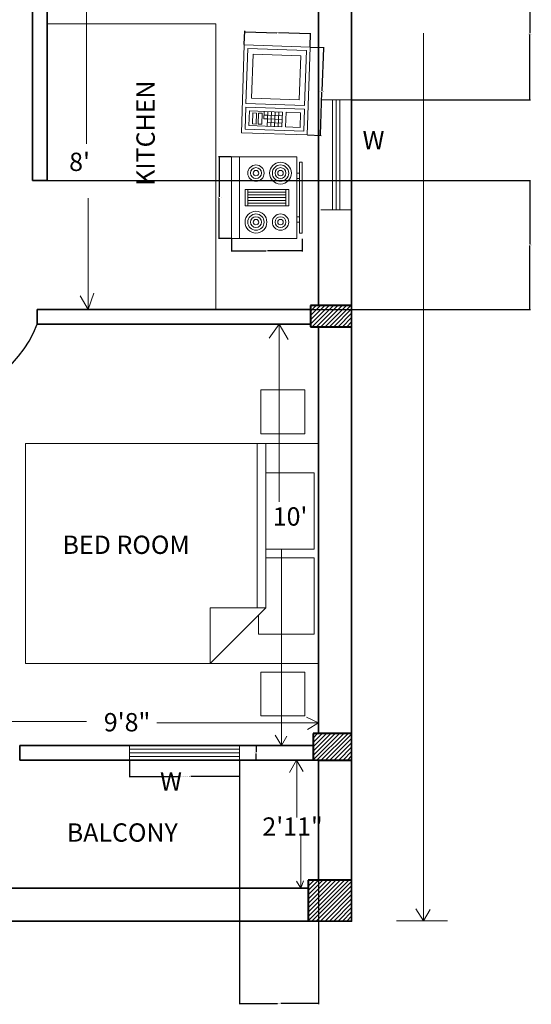
# Model space of a CAD drawing. Units: inches. Extents: x -34 to 385, y -422 to 64.
# Tile 2 of 3: x 246 to 385, y -422 to -153. Entities that reach past the tile are written whole.
import ezdxf

# ---------------------------------------------------------------- set-up
doc = ezdxf.new("R2010")
doc.units = ezdxf.units.IN
doc.header["$MEASUREMENT"] = 0
for name, color, linetype, lineweight in [('A-ANNO-DIMS', 2, 'Continuous', 13), ('A-ANNO-TEXT', 7, 'Continuous', 18), ('A-AREA-IDEN', 7, 'Continuous', 25), ('A-COLS', 1, 'Continuous', 40), ('A-COLS-PATT', 252, 'Continuous', 13), ('A-DOOR', 3, 'Continuous', 25), ('A-EQPM', 8, 'Continuous', 18), ('A-FLOR-CASE', 32, 'Continuous', 20), ('A-FURN', 8, 'Continuous', 18), ('A-GLAZ', 4, 'Continuous', 18), ('A-WALL', 7, 'Continuous', 35)]:
    doc.layers.add(name, color=color, linetype=linetype, lineweight=lineweight)
doc.styles.get("Standard").update_dxf_attribs({"font": 'arial.ttf'})
doc.dimstyles.get("Standard").update_dxf_attribs({"dimtxt": 0.18, "dimasz": 0.18, "dimexe": 0.18, "dimexo": 0.0625, "dimgap": 0.09, "dimtad": 0, "dimtih": 1, "dimtoh": 1, "dimdec": 4, "dimzin": 0, "dimdsep": 46, "dimtxsty": 'Standard', "dimcen": 0.09, "dimadec": 0, "dimazin": 0, "dimtfac": 1, "dimtdec": 4, "dimtofl": 0, "dimtmove": 0, "dimatfit": 3, "dimfxl": 1, "dimtolj": 1, "dimtzin": 0, "dimarcsym": 0})

# ---------------------------------------------------------------- blocks, each defined once
blk = doc.blocks.new('Range-Oven - 30 in top')
for p, q in [((0, -3), (30, -3)), ((12, -6), (18, -6)), ((13, -20), (13, -6)), ((14, -6), (14, -20)), ((15, -20), (15, -6)), ((16, -6), (16, -20)), ((17, -20), (17, -6)), ((18, -20), (12, -20)), ((6, -24), (6, -25)), ((8, -25), (8, -24)), ((22, -25), (22, -24)), ((24, -24), (24, -25))]:
    blk.add_line(p, q)
for points in [[(0, -24), (0, 0), (30, 0), (30, -24)], [(12, -21), (12, -5), (18, -5), (18, -21)], [(2, -26), (2, -25), (28, -25), (28, -26)]]:
    blk.add_lwpolyline(points, close=True)
for centre, radius in [((6, -9), 4), ((6, -9), 3), ((6, -9), 2), ((24, -9), 3), ((24, -9), 2), ((6, -9), 1), ((24, -9), 1), ((24, -18), 4), ((6, -18), 3), ((6, -18), 2), ((6, -18), 1), ((24, -18), 3), ((24, -18), 2), ((24, -18), 1)]:
    blk.add_circle(centre, radius)
blk = doc.blocks.new('Microwave')
for p, q in [((19, 7), (19, 11)), ((20, 11), (20, 7)), ((21, 7), (21, 11)), ((18, 10), (22, 10)), ((22, 9), (18, 9)), ((18, 8), (22, 8)), ((22, 7), (18, 7)), ((20, 6), (18, 6)), ((19, 6), (19, 7)), ((20, 7), (20, 6))]:
    blk.add_line(p, q)
for points in [[(0, 0), (0, 18), (24, 18), (24, 0)], [(1, 1), (1, 17), (16, 17), (16, 1)], [(17, 1), (17, 17), (23, 17), (23, 1)], [(2.5, 2.5), (2.5, 15.5), (14.5, 15.5), (14.5, 2.5)], [(18, 12), (18, 16), (22, 16), (22, 12)], [(18, 2), (18, 11), (22, 11), (22, 2)], [(18.5, 4.5), (18.5, 5.5), (21.5, 5.5), (21.5, 4.5)], [(18.5, 3), (18.5, 4), (21.5, 4), (21.5, 3)]]:
    blk.add_lwpolyline(points, close=True)
blk = doc.blocks.new('Bed - Queen')
for p, q in [((0, -80.00003), (0, 0)), ((0, 0), (59.99999, 0)), ((59.99999, 0), (59.99999, -80.00003)), ((7.99999, -1.2), (28.79998, -1.2)), ((7.99999, -14.4), (7.99999, -1.2)), ((28.79998, -1.2), (28.79998, -14.4)), ((31.19999, -1.2), (51.99999, -1.2)), ((31.19999, -14.4), (31.19999, -1.2)), ((51.99999, -1.2), (51.99999, -16.4)), ((0, -14.4), (44.8, -14.4)), ((59.99999, -29.6), (44.8, -14.4)), ((44.8, -14.4), (44.8, -29.6)), ((44.8, -16.8), (0, -16.8)), ((51.99999, -16.4), (46.79936, -16.4)), ((44.8, -29.6), (59.99999, -29.6)), ((59.99999, -80.00003), (0, -80.00003))]:
    blk.add_line(p, q)
blk = doc.blocks.new('WIN-30IN-4IN-WALL')
for p, q in [((0, 4), (0, 0)), ((0, 3), (30, 3)), ((30, 4), (30, 0)), ((0, 2), (30, 2)), ((0, 1), (30, 1))]:
    blk.add_line(p, q)
blk = doc.blocks.new('NIGHTSTAND-12IN')
blk.add_lwpolyline([(12, 0), (0, 0), (0, 12), (12, 12)], close=True)
blk = doc.blocks.new('*D24')
at = {"layer": 'A-ANNO-DIMS', "color": 0, "lineweight": -2, "transparency": 16777216}
for p, q in [((275.66, -355.21), (275.66, -359.82)), ((305.66, -355.21), (305.66, -359.82)), ((275.84, -359.64), (288.91, -359.64)), ((305.48, -359.64), (292.41, -359.64))]:
    blk.add_line(p, q, dxfattribs=at)
at = {"layer": 'A-ANNO-DIMS', "color": 0, "transparency": 16777216}
for points in [[(275.84, -359.61), (275.84, -359.67), (275.66, -359.64)], [(305.48, -359.61), (305.48, -359.67), (305.66, -359.64)]]:
    blk.add_solid(points, dxfattribs=at)
at = {"layer": 'Defpoints', "color": 0, "transparency": 16777216}
for p in [(275.66, -355.14), (305.66, -355.14), (305.66, -359.64)]:
    blk.add_point(p, dxfattribs=at)
at = {"layer": 'A-ANNO-DIMS', "color": 0, "transparency": 16777216, "insert": (290.66, -359.64), "char_height": 0.18, "attachment_point": 5}
blk.add_mtext('\\A1;BALCONY WINDOW 30 TYP.', dxfattribs=at)
blk = doc.blocks.new('*D25')
at = {"layer": 'A-ANNO-DIMS', "color": 0, "lineweight": -2, "transparency": 16777216}
for p, q in [((305.72, -351.14), (310.34, -351.14)), ((310.16, -351.32), (310.16, -352.96)), ((310.16, -354.96), (310.16, -353.32)), ((305.72, -355.14), (310.34, -355.14))]:
    blk.add_line(p, q, dxfattribs=at)
at = {"layer": 'A-ANNO-DIMS', "color": 0, "transparency": 16777216}
for points in [[(310.13, -351.32), (310.19, -351.32), (310.16, -351.14)], [(310.13, -354.96), (310.19, -354.96), (310.16, -355.14)]]:
    blk.add_solid(points, dxfattribs=at)
at = {"layer": 'Defpoints', "color": 0, "transparency": 16777216}
for p in [(305.66, -351.14), (310.16, -351.14), (305.66, -355.14)]:
    blk.add_point(p, dxfattribs=at)
at = {"layer": 'A-ANNO-DIMS', "color": 0, "transparency": 16777216, "insert": (310.16, -353.14), "char_height": 0.18, "attachment_point": 5}
blk.add_mtext('\\A1;4 TYP.', dxfattribs=at)
blk = doc.blocks.new('*D28')
at = {"layer": 'A-ANNO-DIMS', "color": 0, "lineweight": -2, "transparency": 16777216}
for p, q in [((325.01, -160.49), (328.73, -160.61)), ((328.54, -160.79), (328.15, -172.42)), ((327.75, -184.41), (328.14, -172.78)), ((324.21, -184.47), (327.92, -184.6))]:
    blk.add_line(p, q, dxfattribs=at)
at = {"layer": 'A-ANNO-DIMS', "color": 0, "transparency": 16777216}
for points in [[(328.51, -160.79), (328.57, -160.79), (328.55, -160.61)], [(327.72, -184.41), (327.78, -184.41), (327.74, -184.59)]]:
    blk.add_solid(points, dxfattribs=at)
at = {"layer": 'Defpoints', "color": 0, "transparency": 16777216}
for p in [(324.95, -160.49), (324.15, -184.47), (327.74, -184.59)]:
    blk.add_point(p, dxfattribs=at)
at = {"layer": 'A-ANNO-DIMS', "color": 0, "transparency": 16777216, "insert": (328.15, -172.6), "char_height": 0.18, "attachment_point": 5}
blk.add_mtext('\\A1;MICROWAVE 24', dxfattribs=at)
blk = doc.blocks.new('*D29')
at = {"layer": 'A-ANNO-DIMS', "color": 0, "lineweight": -2, "transparency": 16777216}
for p, q in [((306.96, -159.82), (307.09, -156.1)), ((307.26, -156.29), (315.87, -156.58)), ((324.89, -156.88), (316.29, -156.59)), ((324.95, -160.42), (325.08, -156.71))]:
    blk.add_line(p, q, dxfattribs=at)
at = {"layer": 'A-ANNO-DIMS', "color": 0, "transparency": 16777216}
for points in [[(307.26, -156.26), (307.26, -156.32), (307.08, -156.28)], [(324.89, -156.85), (324.89, -156.91), (325.07, -156.89)]]:
    blk.add_solid(points, dxfattribs=at)
at = {"layer": 'Defpoints', "color": 0, "transparency": 16777216}
for p in [(325.07, -156.89), (306.96, -159.88), (324.95, -160.49)]:
    blk.add_point(p, dxfattribs=at)
at = {"layer": 'A-ANNO-DIMS', "color": 0, "transparency": 16777216, "insert": (316.08, -156.59), "char_height": 0.18, "attachment_point": 5}
blk.add_mtext('\\A1;18', dxfattribs=at)
blk = doc.blocks.new('*D30')
at = {"layer": 'A-ANNO-DIMS', "color": 0, "lineweight": -2, "transparency": 16777216}
for p, q in [((303.4, -190.44), (299.94, -190.44)), ((300.12, -190.62), (300.12, -201.41)), ((300.12, -212.56), (300.12, -201.77)), ((303.4, -212.74), (299.94, -212.74))]:
    blk.add_line(p, q, dxfattribs=at)
at = {"layer": 'A-ANNO-DIMS', "color": 0, "transparency": 16777216}
for points in [[(300.09, -190.62), (300.15, -190.62), (300.12, -190.44)], [(300.09, -212.56), (300.15, -212.56), (300.12, -212.74)]]:
    blk.add_solid(points, dxfattribs=at)
at = {"layer": 'Defpoints', "color": 0, "transparency": 16777216}
for p in [(300.12, -190.44), (303.47, -190.44), (303.47, -212.74)]:
    blk.add_point(p, dxfattribs=at)
at = {"layer": 'A-ANNO-DIMS', "color": 0, "transparency": 16777216, "insert": (300.12, -201.59), "char_height": 0.18, "attachment_point": 5}
blk.add_mtext('\\A1;RANGE 22', dxfattribs=at)
blk = doc.blocks.new('*D31')
at = {"layer": 'A-ANNO-DIMS', "color": 0, "lineweight": -2, "transparency": 16777216}
for p, q in [((303.47, -212.8), (303.47, -216.27)), ((322.8, -212.8), (322.8, -216.27)), ((303.65, -216.09), (312.92, -216.09)), ((322.62, -216.09), (313.34, -216.09))]:
    blk.add_line(p, q, dxfattribs=at)
at = {"layer": 'A-ANNO-DIMS', "color": 0, "transparency": 16777216}
for points in [[(303.65, -216.06), (303.65, -216.12), (303.47, -216.09)], [(322.62, -216.06), (322.62, -216.12), (322.8, -216.09)]]:
    blk.add_solid(points, dxfattribs=at)
at = {"layer": 'Defpoints', "color": 0, "transparency": 16777216}
for p in [(303.47, -212.74), (322.8, -212.74), (303.47, -216.09)]:
    blk.add_point(p, dxfattribs=at)
at = {"layer": 'A-ANNO-DIMS', "color": 0, "transparency": 16777216, "insert": (313.13, -216.09), "char_height": 0.18, "attachment_point": 5}
blk.add_mtext('\\A1;19', dxfattribs=at)
blk = doc.blocks.new('*D37')
at = {"layer": 'A-ANNO-DIMS', "color": 0, "lineweight": -2, "transparency": 16777216}
for p, q in [((336.32, -138.89), (385.11, -138.89)), ((384.93, -139.07), (384.93, -156.71)), ((384.93, -174.71), (384.93, -157.07)), ((336.32, -174.89), (385.11, -174.89))]:
    blk.add_line(p, q, dxfattribs=at)
at = {"layer": 'A-ANNO-DIMS', "color": 0, "transparency": 16777216}
for points in [[(384.9, -139.07), (384.96, -139.07), (384.93, -138.89)], [(384.9, -174.71), (384.96, -174.71), (384.93, -174.89)]]:
    blk.add_solid(points, dxfattribs=at)
at = {"layer": 'Defpoints', "color": 0, "transparency": 16777216}
for p in [(336.26, -138.89), (336.26, -174.89), (384.93, -174.89)]:
    blk.add_point(p, dxfattribs=at)
at = {"layer": 'A-ANNO-DIMS', "color": 0, "transparency": 16777216, "insert": (384.93, -156.89), "char_height": 0.18, "attachment_point": 5}
blk.add_mtext('\\A1;35.995', dxfattribs=at)
blk = doc.blocks.new('*D41')
at = {"layer": 'A-ANNO-DIMS', "color": 0, "lineweight": -2, "transparency": 16777216}
for p, q in [((305.66, -355.21), (305.66, -421.82)), ((327.26, -355.21), (327.26, -421.82)), ((305.84, -421.64), (315.99, -421.64)), ((327.08, -421.64), (316.92, -421.64))]:
    blk.add_line(p, q, dxfattribs=at)
at = {"layer": 'A-ANNO-DIMS', "color": 0, "transparency": 16777216}
for points in [[(305.84, -421.61), (305.84, -421.67), (305.66, -421.64)], [(327.08, -421.61), (327.08, -421.67), (327.26, -421.64)]]:
    blk.add_solid(points, dxfattribs=at)
at = {"layer": 'Defpoints', "color": 0, "transparency": 16777216}
for p in [(305.66, -355.14), (327.26, -355.14), (327.26, -421.64)]:
    blk.add_point(p, dxfattribs=at)
at = {"layer": 'A-ANNO-DIMS', "color": 0, "transparency": 16777216, "insert": (316.46, -421.64), "char_height": 0.18, "attachment_point": 5}
blk.add_mtext('\\A1;21.598', dxfattribs=at)
blk = doc.blocks.new('*D42')
at = {"layer": 'A-ANNO-DIMS', "color": 0, "lineweight": -2, "transparency": 16777216}
for p, q in [((253.23, -196.9), (385.11, -196.9)), ((384.93, -197.08), (384.93, -214.34)), ((384.93, -231.96), (384.93, -214.7)), ((250.46, -232.14), (385.11, -232.14))]:
    blk.add_line(p, q, dxfattribs=at)
at = {"layer": 'A-ANNO-DIMS', "color": 0, "transparency": 16777216}
for points in [[(384.9, -197.08), (384.96, -197.08), (384.93, -196.9)], [(384.9, -231.96), (384.96, -231.96), (384.93, -232.14)]]:
    blk.add_solid(points, dxfattribs=at)
at = {"layer": 'Defpoints', "color": 0, "transparency": 16777216}
for p in [(253.17, -196.9), (250.4, -232.14), (384.93, -232.14)]:
    blk.add_point(p, dxfattribs=at)
at = {"layer": 'A-ANNO-DIMS', "color": 0, "transparency": 16777216, "insert": (384.93, -214.52), "char_height": 0.18, "attachment_point": 5}
blk.add_mtext('\\A1;35.244', dxfattribs=at)

msp = doc.modelspace()

# ---------------------------------------------------------------- hatches: boundary and pattern name
at = {"layer": 'A-COLS-PATT'}
h = msp.add_hatch(dxfattribs=at)
h.set_pattern_fill('ANSI31', color=256, scale=6.7)
h.set_pattern_definition([(45, (-1587.6103, -800.894), (-0.59220193, 0.59220193), [])])
h.paths.add_polyline_path([(34.5325, 20.857), (24.2567, 20.857), (24.2567, 10.5552), (34.5325, 10.5552)])
h.paths.add_polyline_path([(155.6882, 20.857), (147.6505, 20.857), (147.6505, 8.8355), (155.6882, 8.8355)])
h.paths.add_polyline_path([(214.1102, 20.857), (204.3358, 20.857), (204.3358, 9.8804), (214.1102, 9.8804)])
h.paths.add_polyline_path([(336.2567, 20.857), (324.9664, 20.857), (324.9664, 9.4113), (336.2567, 9.4113)])
h.paths.add_polyline_path([(336.2567, -129.6656), (324.4892, -129.6656), (324.4892, -138.8931), (336.2567, -138.8931)])
h.paths.add_polyline_path([(212.9763, -130.7216), (204.8831, -130.7216), (204.8831, -136.143), (212.9763, -136.143)])
h.paths.add_polyline_path([(154.6774, -130.7571), (147.9004, -130.7571), (147.9004, -136.143), (154.6774, -136.143)])
h.paths.add_polyline_path([(36.3503, -129.7825), (24.2567, -129.7825), (24.2567, -139.3836), (36.3503, -139.3836)])
h.paths.add_polyline_path([(35.9496, -230.9729), (24.2567, -230.9729), (24.2567, -238.1404), (35.9496, -238.1404)])
h.paths.add_polyline_path([(153.2567, -232.143), (148.2796, -232.143), (148.2796, -237.1221), (148.2796, -237.5145), (153.2567, -237.5145)])
h.paths.add_polyline_path([(212.7, -232.143), (207.2567, -232.143), (207.2567, -238.4312), (212.7, -238.4312)])
h.paths.add_polyline_path([(336.2567, -230.9985), (325.0216, -230.9985), (325.0216, -236.8618), (336.2567, -236.8618)])
h.paths.add_polyline_path([(34.6412, -348.0183), (24.2567, -348.0183), (24.2567, -355.143), (33.2567, -355.143), (34.6412, -355.143)])
h.paths.add_polyline_path([(35.0834, -388.1327), (24.2567, -388.1327), (24.2567, -399.143), (35.0834, -399.143)])
h.paths.add_polyline_path([(156.485, -388.1078), (149.2567, -388.1078), (149.2567, -390.143), (149.2567, -399.143), (156.485, -399.143)])
h.paths.add_polyline_path([(153.2567, -351.143), (148.4284, -351.143), (148.4284, -355.9617), (153.2567, -355.9617)])
h.paths.add_polyline_path([(211.2567, -390.143), (211.2567, -388.2391), (204.1967, -388.2391), (204.1967, -399.143), (211.2567, -399.143)])
h.paths.add_polyline_path([(213.2403, -351.143), (207.2567, -351.143), (207.2567, -356.6203), (213.2403, -356.6203)])
h.paths.add_polyline_path([(336.2567, -347.847), (325.718, -347.847), (325.718, -355.143), (327.2567, -355.143), (336.2567, -355.143)])
h.paths.add_polyline_path([(336.2567, -387.9228), (324.3995, -387.9228), (324.3995, -399.143), (336.2567, -399.143)])

# ---------------------------------------------------------------- linework, layer by layer
at = {"layer": 'A-ANNO-DIMS'}
for p, q in [((263.8812, -136.143), (263.8812, -186.9196)), ((355.9176, -156.6786), (355.9176, -399.143)), ((264.3365, -201.7704), (264.3365, -232.143)), ((262.1293, -228.3967), (264.3365, -232.143)), ((264.3365, -232.143), (265.9389, -227.6693)), ((313.7112, -239.9906), (316.4725, -236.143)), ((316.4725, -236.143), (316.4725, -284.6021)), ((316.4725, -236.143), (318.8982, -240.3444)), ((317.1348, -297.5403), (317.1348, -351.143)), ((323.952, -343.4634), (327.2567, -345.0039)), ((211.2567, -344.6286), (263.9083, -344.6286)), ((283.0749, -345.0039), (327.2567, -345.0039)), ((327.2567, -345.0039), (324.1796, -346.7805)), ((315.3854, -348.3126), (317.1348, -351.143)), ((317.1348, -351.143), (318.6106, -348.5869)), ((319.2708, -358.5338), (321.2285, -355.143)), ((321.2285, -355.143), (323.0361, -358.2738)), ((321.3115, -355.143), (321.3115, -370.7981)), ((322.383, -375.8186), (322.383, -390.143)), ((321.2569, -388.2397), (322.383, -390.143)), ((322.383, -390.143), (323.1607, -388.129)), ((353.8171, -395.7977), (355.9176, -399.0434)), ((355.9176, -399.0434), (357.7351, -395.8955)), ((348.4721, -399.0434), (362.4295, -399.0434))]:
    msp.add_line(p, q, dxfattribs=at)
at = {"layer": 'A-COLS'}
for p, q in [((336.2567, -230.9985), (325.0216, -230.9985)), ((325.0216, -230.9985), (325.0216, -236.8618)), ((325.0216, -236.8618), (336.2567, -236.8618)), ((336.2567, -347.847), (325.718, -347.847)), ((325.718, -347.847), (325.718, -355.143)), ((327.2567, -355.143), (336.2567, -355.143)), ((336.2567, -387.9228), (324.3995, -387.9228)), ((324.3995, -387.9228), (324.3995, -399.143))]:
    msp.add_line(p, q, dxfattribs=at)
at = {"layer": 'A-DOOR'}
msp.add_arc((221.4774, -225.3071), 30.8836, 264.92528, 339.459894, dxfattribs=at)
at = {"layer": 'A-FLOR-CASE'}
for p, q in [((253.1677, -154.115), (299.2041, -154.115)), ((299.2041, -154.115), (299.2041, -232.143))]:
    msp.add_line(p, q, dxfattribs=at)
at = {"layer": 'A-GLAZ'}
for p, q in [((327.8171, -174.8878), (336.2567, -174.8878)), ((331.0369, -174.8878), (331.0369, -204.8878)), ((332.0369, -174.8878), (332.0369, -204.8878)), ((333.0369, -174.8878), (333.0369, -204.8878)), ((327.8171, -204.8878), (336.2567, -204.8878))]:
    msp.add_line(p, q, dxfattribs=at)
at = {"layer": 'A-WALL'}
for p, q in [((253.1677, -196.8987), (253.1677, -132.143)), ((249.1677, -136.143), (249.1677, -196.8987)), ((327.2567, -138.8931), (327.2567, -230.9985)), ((249.1677, -196.8987), (253.1677, -196.8987)), ((250.3976, -232.143), (250.3976, -236.143)), ((250.3976, -232.143), (325.0216, -232.143)), ((250.3976, -236.143), (325.0216, -236.143)), ((327.2567, -236.8618), (327.2567, -347.847)), ((325.718, -351.143), (245.659, -351.143)), ((245.659, -351.143), (245.659, -355.143)), ((327.2567, -355.143), (245.659, -355.143)), ((327.2567, -355.143), (327.2567, -387.9228)), ((324.3995, -390.143), (211.2567, -390.143))]:
    msp.add_line(p, q, dxfattribs=at)
msp.add_lwpolyline([(24.2567, 20.857), (336.2567, 20.857), (336.2567, -399.143), (24.2567, -399.143)], close=True, dxfattribs=at)

# ---------------------------------------------------------------- block references
at = {"layer": 'A-EQPM', "rotation": 268.0777171535374}
msp.add_blockref('Microwave', (306.9611, -159.8817), dxfattribs=at)
at = {"layer": 'A-EQPM', "xscale": 0.7434357738590788, "yscale": 0.7434357738590788, "zscale": 0.7434357738590788, "rotation": 90}
msp.add_blockref('Range-Oven - 30 in top', (303.4659, -212.741), dxfattribs=at)
at = {"layer": 'A-FURN'}
for p in [(311.451, -266.075), (311.451, -343.1064)]:
    msp.add_blockref('NIGHTSTAND-12IN', p, dxfattribs=at)
at = {"layer": 'A-FURN', "rotation": 270}
msp.add_blockref('Bed - Queen', (327.2567, -268.7403), dxfattribs=at)
at = {"layer": 'A-GLAZ'}
msp.add_blockref('WIN-30IN-4IN-WALL', (275.659, -355.143), dxfattribs=at)

# ---------------------------------------------------------------- texts
at = {"layer": 'A-ANNO-DIMS', "char_height": 5, "attachment_point": 1}
for s, width, insert in [("8'", 11.131015, (259.1567, -189.3175)), ("10'", 6.501124, (314.7226, -286.1383)), ('9\'8"', 24.448319, (268.6166, -342.3071)), ('2\'11"', 7.143648, (311.898, -370.7981))]:
    msp.add_mtext_dynamic_manual_height_columns(s, width=width, gutter_width=25, heights=[0], dxfattribs=dict(at, insert=insert))
at = {"layer": 'A-ANNO-TEXT', "char_height": 5, "attachment_point": 1}
for width, insert in [(10.234455, (339.2372, -183.3616)), (13.50209, (283.9535, -358.4693))]:
    msp.add_mtext_dynamic_manual_height_columns('W', width=width, gutter_width=25, heights=[0], dxfattribs=dict(at, insert=insert))
at = {"layer": 'A-AREA-IDEN', "insert": (277.5189, -198.3689), "char_height": 5, "attachment_point": 1, "rotation": 90}
msp.add_mtext_dynamic_manual_height_columns('KITCHEN', width=32.24355, gutter_width=25, heights=[0], dxfattribs=at)
at = {"layer": 'A-AREA-IDEN', "char_height": 5, "attachment_point": 1}
for s, width, insert in [('BED ROOM', 39.759385, (257.3561, -293.8675)), ('BALCONY', 50.318627, (258.5166, -372.4254))]:
    msp.add_mtext_dynamic_manual_height_columns(s, width=width, gutter_width=25, heights=[0], dxfattribs=dict(at, insert=insert))

# ---------------------------------------------------------------- dimensions: what is measured, and where the dimension line sits
at = {"layer": 'A-ANNO-DIMS'}
for base, p1, p2, angle, override, picture, middle in [((384.9295, -174.8878), (336.2567, -138.8931), (336.2567, -174.8878), 90, {"dimdec": 3, "dimlfac": 1, "dimrnd": 0, "dimzin": 0, "dimdsep": 46, "dimlunit": 2}, '*D37', (384.9295, -156.8905)), ((325.0717, -156.8875), (306.9611, -159.8817), (324.951, -160.4854), 358.077717, {"dimdec": 0, "dimlfac": 1, "dimrnd": 0, "dimzin": 0, "dimdsep": 46, "dimlunit": 2}, '*D29', (316.0768, -156.5856)), ((384.9295, -232.143), (253.1677, -196.8987), (250.3976, -232.143), 90, {"dimdec": 3, "dimlfac": 1, "dimrnd": 0, "dimzin": 0, "dimdsep": 46, "dimlunit": 2}, '*D42', (384.9295, -214.5209)), ((303.4659, -216.0865), (322.7952, -212.741), (303.4659, -212.741), 180, {"dimdec": 0, "dimlfac": 1, "dimrnd": 0, "dimzin": 0, "dimdsep": 46, "dimlunit": 2}, '*D31', (313.1306, -216.0865))]:
    dim = msp.add_linear_dim(base=base, p1=p1, p2=p2, angle=angle, dimstyle='Standard', override=override, dxfattribs=at)
    dim.commit()
    dim.dimension.update_dxf_attribs({"geometry": picture, "text_midpoint": middle})
for base, p1, p2, angle, text, picture, middle in [((327.7439, -184.5927), (324.951, -160.4854), (324.1459, -184.4719), 268.077717, 'MICROWAVE <>', '*D28', (328.1464, -172.5995)), ((300.1205, -190.438), (303.4659, -212.741), (303.4659, -190.438), 90, 'RANGE <>', '*D30', (300.1205, -201.5895)), ((310.159, -351.143), (305.659, -355.143), (305.659, -351.143), 90, '<> TYP.', '*D25', (310.159, -353.143))]:
    dim = msp.add_linear_dim(base=base, p1=p1, p2=p2, angle=angle, text=text, dimstyle='Standard', override={"dimdec": 0, "dimlfac": 1, "dimrnd": 0, "dimzin": 0, "dimdsep": 46, "dimlunit": 2}, dxfattribs=at)
    dim.commit()
    dim.dimension.update_dxf_attribs({"geometry": picture, "text_midpoint": middle})
dim = msp.add_linear_dim(base=(305.659, -359.643), p1=(275.659, -355.143), p2=(305.659, -355.143), text='BALCONY WINDOW <> TYP.', dimstyle='Standard', override={"dimdec": 0, "dimlfac": 1, "dimrnd": 0, "dimzin": 0, "dimdsep": 46, "dimlunit": 2}, dxfattribs=at)
dim.commit()
dim.dimension.update_dxf_attribs({"geometry": '*D24', "text_midpoint": (290.659, -359.643)})
dim = msp.add_linear_dim(base=(327.2567, -421.643), p1=(305.659, -355.143), p2=(327.2567, -355.143), dimstyle='Standard', override={"dimdec": 3, "dimlfac": 1, "dimrnd": 0, "dimzin": 0, "dimdsep": 46, "dimlunit": 2}, dxfattribs=at)
dim.commit()
dim.dimension.update_dxf_attribs({"geometry": '*D41', "text_midpoint": (316.4578, -421.643)})

doc.saveas('drawing.dxf')
